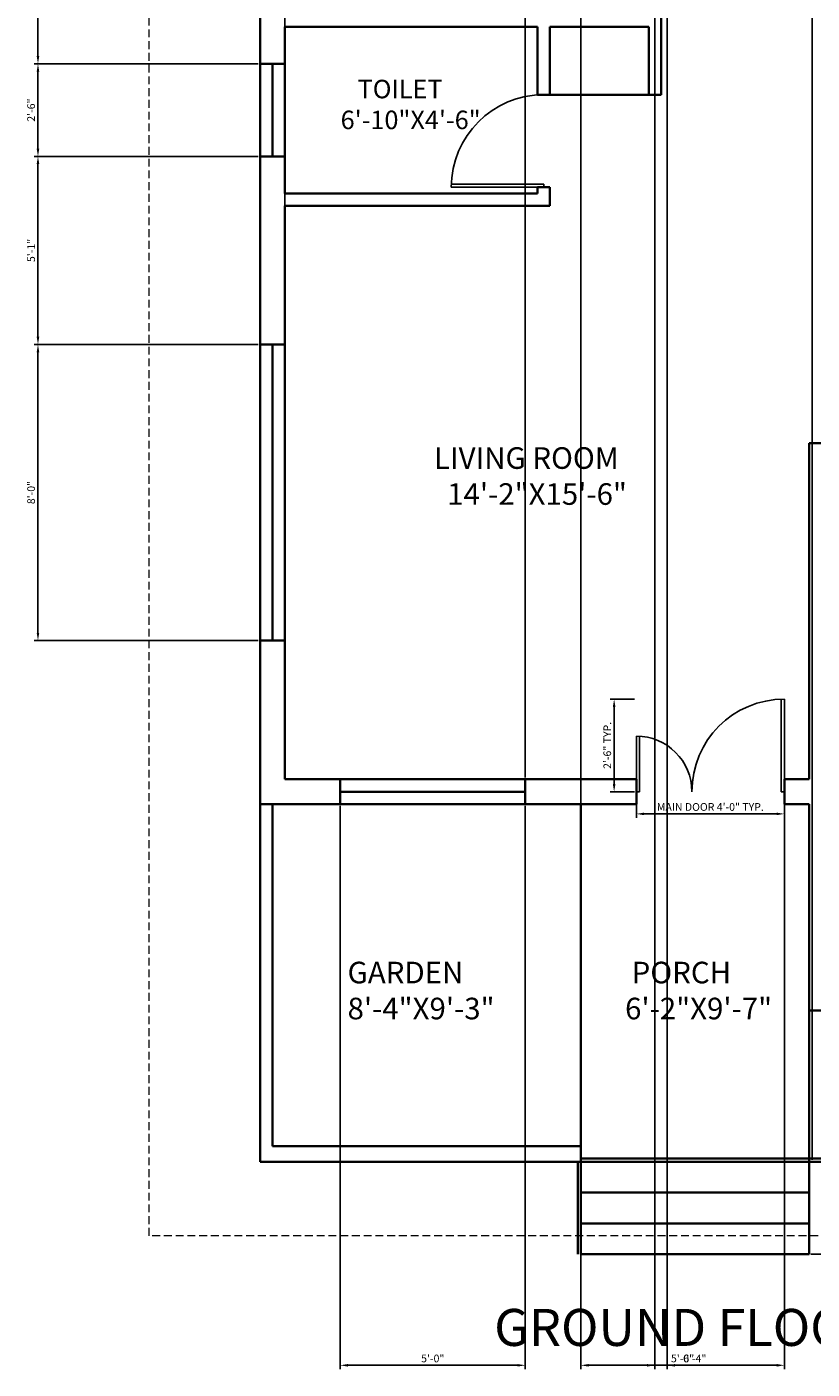
# Model space of a CAD drawing. Units: inches. Extents: x 1566 to 2546, y 1087 to 2705.
# Tile 24 of 27: x 1566 to 1821, y 1974 to 2409. Entities that reach past the tile are written whole.
import ezdxf

# ---------------------------------------------------------------- set-up
doc = ezdxf.new("R2010")
doc.units = ezdxf.units.IN
doc.linetypes.add('DASHED', pattern=[19.05, 12.7, -6.35])
for name, color, linetype, lineweight in [('A-ANNO-DIMS', 2, 'Continuous', 18), ('A-AREA-IDEN', 7, 'Continuous', 18), ('A-DOOR', 4, 'Continuous', 25), ('A-FLOR-OVHD', 8, 'DASHED', 18), ('A-WALL', 7, 'Continuous', 35)]:
    doc.layers.add(name, color=color, linetype=linetype, lineweight=lineweight)
doc.styles.get("Standard").update_dxf_attribs({"font": 'arial.ttf'})
doc.dimstyles.new('ISO-25', dxfattribs={"dimtxt": 2.5, "dimasz": 2.5, "dimexe": 1.25, "dimexo": 0.625, "dimtad": 1, "dimtxsty": 'Standard', "dimcen": 2.5, "dimadec": 0, "dimazin": 0, "dimtfac": 1, "dimtmove": 0, "dimatfit": 3, "dimfxl": 1, "dimarcsym": 0})

# ---------------------------------------------------------------- blocks, each defined once
blk = doc.blocks.new('d2')
for p, q in [((3364.08, 1632.29), (3364.08, 1602.29)), ((3365.08, 1632.29), (3365.08, 1602.29)), ((3364.08, 1602.29), (3365.08, 1602.29))]:
    blk.add_line(p, q)
at = {"ltscale": 0.3}
blk.add_arc((3364.08, 1602.29), 30, 0, 90, dxfattribs=at)
blk = doc.blocks.new('MD')
for p, q in [((1753.46, 1293.03), (1753.46, 1323.03)), ((1754.46, 1293.03), (1754.46, 1323.03)), ((1800.46, 1293.03), (1800.46, 1311.03)), ((1801.46, 1293.03), (1801.46, 1311.03)), ((1753.46, 1293.03), (1754.46, 1293.03)), ((1800.46, 1293.03), (1801.46, 1293.03))]:
    blk.add_line(p, q)
at = {"ltscale": 0.3}
for centre, radius, start, end in [((1753.46, 1293.03), 30, 0, 90), ((1801.46, 1293.03), 18, 90, 180)]:
    blk.add_arc(centre, radius, start, end, dxfattribs=at)
blk = doc.blocks.new('*D39')
at = {"layer": 'A-ANNO-DIMS', "color": 0, "lineweight": -2, "transparency": 16777216}
for p, q in [((1763.53, 2160.72), (1763.53, 2152.9)), ((1811.53, 2160.72), (1811.53, 2152.9)), ((1809.03, 2154.15), (1766.03, 2154.15))]:
    blk.add_line(p, q, dxfattribs=at)
at = {"layer": 'A-ANNO-DIMS', "color": 0, "transparency": 16777216}
for points in [[(1766.03, 2154.56), (1766.03, 2153.73), (1763.53, 2154.15)], [(1809.03, 2154.56), (1809.03, 2153.73), (1811.53, 2154.15)]]:
    blk.add_solid(points, dxfattribs=at)
at = {"layer": 'Defpoints', "color": 0, "transparency": 16777216}
for p in [(1763.53, 2161.35), (1811.53, 2161.35), (1763.53, 2154.15)]:
    blk.add_point(p, dxfattribs=at)
at = {"layer": 'A-ANNO-DIMS', "color": 0, "transparency": 16777216, "insert": (1787.53, 2156.07), "char_height": 2.5, "attachment_point": 5}
blk.add_mtext('MAIN DOOR 4\'-0" TYP.', dxfattribs=at)
blk = doc.blocks.new('*D40')
at = {"layer": 'A-ANNO-DIMS', "color": 0, "lineweight": -2, "transparency": 16777216}
for p, q in [((1762.9, 2191.35), (1755.08, 2191.35)), ((1756.33, 2163.85), (1756.33, 2188.85)), ((1762.9, 2161.35), (1755.08, 2161.35))]:
    blk.add_line(p, q, dxfattribs=at)
at = {"layer": 'A-ANNO-DIMS', "color": 0, "transparency": 16777216}
for points in [[(1755.91, 2188.85), (1756.75, 2188.85), (1756.33, 2191.35)], [(1755.91, 2163.85), (1756.75, 2163.85), (1756.33, 2161.35)]]:
    blk.add_solid(points, dxfattribs=at)
at = {"layer": 'Defpoints', "color": 0, "transparency": 16777216}
for p in [(1756.33, 2191.35), (1763.53, 2191.35), (1763.53, 2161.35)]:
    blk.add_point(p, dxfattribs=at)
at = {"layer": 'A-ANNO-DIMS', "color": 0, "transparency": 16777216, "insert": (1754.43, 2176.35), "char_height": 2.5, "attachment_point": 5, "rotation": 90}
blk.add_mtext('2\'-6" TYP.', dxfattribs=at)
blk = doc.blocks.new('*D70')
at = {"layer": 'A-ANNO-DIMS', "color": 0, "lineweight": -2, "transparency": 16777216}
for p, q in [((1769.53, 2656.72), (1769.53, 1974.1)), ((1773.53, 2656.72), (1773.53, 1974.1)), ((1767.03, 1975.35), (1764.53, 1975.35)), ((1769.53, 1975.35), (1773.53, 1975.35)), ((1776.03, 1975.35), (1786.43, 1975.35))]:
    blk.add_line(p, q, dxfattribs=at)
at = {"layer": 'A-ANNO-DIMS', "color": 0, "transparency": 16777216}
for points in [[(1767.03, 1975.76), (1767.03, 1974.93), (1769.53, 1975.35)], [(1776.03, 1975.76), (1776.03, 1974.93), (1773.53, 1975.35)]]:
    blk.add_solid(points, dxfattribs=at)
at = {"layer": 'Defpoints', "color": 0, "transparency": 16777216}
for p in [(1769.53, 2657.35), (1773.53, 2657.35), (1773.53, 1975.35)]:
    blk.add_point(p, dxfattribs=at)
at = {"layer": 'A-ANNO-DIMS', "color": 0, "transparency": 16777216, "insert": (1782.48, 1977.25), "char_height": 2.5, "attachment_point": 5}
blk.add_mtext('0\'-4"', dxfattribs=at)
blk = doc.blocks.new('*D75')
at = {"layer": 'A-ANNO-DIMS', "color": 0, "lineweight": -2, "transparency": 16777216}
for p, q in [((1640.9, 2437.35), (1568.28, 2437.35)), ((1569.53, 2434.85), (1569.53, 2399.85)), ((1640.9, 2397.35), (1568.28, 2397.35))]:
    blk.add_line(p, q, dxfattribs=at)
at = {"layer": 'A-ANNO-DIMS', "color": 0, "transparency": 16777216}
for points in [[(1569.11, 2434.85), (1569.95, 2434.85), (1569.53, 2437.35)], [(1569.11, 2399.85), (1569.95, 2399.85), (1569.53, 2397.35)]]:
    blk.add_solid(points, dxfattribs=at)
at = {"layer": 'Defpoints', "color": 0, "transparency": 16777216}
for p in [(1641.53, 2437.35), (1569.53, 2397.35), (1641.53, 2397.35)]:
    blk.add_point(p, dxfattribs=at)
at = {"layer": 'A-ANNO-DIMS', "color": 0, "transparency": 16777216, "insert": (1567.63, 2417.35), "char_height": 2.5, "attachment_point": 5, "rotation": 90}
blk.add_mtext('3\'-4"', dxfattribs=at)
blk = doc.blocks.new('*D76')
at = {"layer": 'A-ANNO-DIMS', "color": 0, "lineweight": -2, "transparency": 16777216}
for p, q in [((1640.9, 2397.35), (1568.28, 2397.35)), ((1569.53, 2394.85), (1569.53, 2369.85)), ((1640.9, 2367.35), (1568.28, 2367.35))]:
    blk.add_line(p, q, dxfattribs=at)
at = {"layer": 'A-ANNO-DIMS', "color": 0, "transparency": 16777216}
for points in [[(1569.11, 2394.85), (1569.95, 2394.85), (1569.53, 2397.35)], [(1569.11, 2369.85), (1569.95, 2369.85), (1569.53, 2367.35)]]:
    blk.add_solid(points, dxfattribs=at)
at = {"layer": 'Defpoints', "color": 0, "transparency": 16777216}
for p in [(1641.53, 2397.35), (1569.53, 2367.35), (1641.53, 2367.35)]:
    blk.add_point(p, dxfattribs=at)
at = {"layer": 'A-ANNO-DIMS', "color": 0, "transparency": 16777216, "insert": (1567.63, 2382.35), "char_height": 2.5, "attachment_point": 5, "rotation": 90}
blk.add_mtext('2\'-6"', dxfattribs=at)
blk = doc.blocks.new('*D77')
at = {"layer": 'A-ANNO-DIMS', "color": 0, "lineweight": -2, "transparency": 16777216}
for p, q in [((1640.9, 2367.35), (1568.28, 2367.35)), ((1569.53, 2364.85), (1569.53, 2308.85)), ((1640.9, 2306.35), (1568.28, 2306.35))]:
    blk.add_line(p, q, dxfattribs=at)
at = {"layer": 'A-ANNO-DIMS', "color": 0, "transparency": 16777216}
for points in [[(1569.11, 2364.85), (1569.95, 2364.85), (1569.53, 2367.35)], [(1569.11, 2308.85), (1569.95, 2308.85), (1569.53, 2306.35)]]:
    blk.add_solid(points, dxfattribs=at)
at = {"layer": 'Defpoints', "color": 0, "transparency": 16777216}
for p in [(1641.53, 2367.35), (1569.53, 2306.35), (1641.53, 2306.35)]:
    blk.add_point(p, dxfattribs=at)
at = {"layer": 'A-ANNO-DIMS', "color": 0, "transparency": 16777216, "insert": (1567.63, 2336.85), "char_height": 2.5, "attachment_point": 5, "rotation": 90}
blk.add_mtext('5\'-1"', dxfattribs=at)
blk = doc.blocks.new('*D78')
at = {"layer": 'A-ANNO-DIMS', "color": 0, "lineweight": -2, "transparency": 16777216}
for p, q in [((1640.9, 2306.35), (1568.28, 2306.35)), ((1569.53, 2303.85), (1569.53, 2212.85)), ((1640.9, 2210.35), (1568.28, 2210.35))]:
    blk.add_line(p, q, dxfattribs=at)
at = {"layer": 'A-ANNO-DIMS', "color": 0, "transparency": 16777216}
for points in [[(1569.11, 2303.85), (1569.95, 2303.85), (1569.53, 2306.35)], [(1569.11, 2212.85), (1569.95, 2212.85), (1569.53, 2210.35)]]:
    blk.add_solid(points, dxfattribs=at)
at = {"layer": 'Defpoints', "color": 0, "transparency": 16777216}
for p in [(1641.53, 2306.35), (1569.53, 2210.35), (1641.53, 2210.35)]:
    blk.add_point(p, dxfattribs=at)
at = {"layer": 'A-ANNO-DIMS', "color": 0, "transparency": 16777216, "insert": (1567.63, 2258.35), "char_height": 2.5, "attachment_point": 5, "rotation": 90}
blk.add_mtext('8\'-0"', dxfattribs=at)
blk = doc.blocks.new('*D79')
at = {"layer": 'A-ANNO-DIMS', "color": 0, "lineweight": -2, "transparency": 16777216}
for p, q in [((1649.53, 2165.97), (1649.53, 2702.6)), ((1652.03, 2701.35), (1725.03, 2701.35)), ((1727.53, 2165.97), (1727.53, 2702.6))]:
    blk.add_line(p, q, dxfattribs=at)
at = {"layer": 'A-ANNO-DIMS', "color": 0, "transparency": 16777216}
for points in [[(1652.03, 2701.76), (1652.03, 2700.93), (1649.53, 2701.35)], [(1725.03, 2701.76), (1725.03, 2700.93), (1727.53, 2701.35)]]:
    blk.add_solid(points, dxfattribs=at)
at = {"layer": 'Defpoints', "color": 0, "transparency": 16777216}
for p in [(1727.53, 2701.35), (1649.53, 2165.35), (1727.53, 2165.35)]:
    blk.add_point(p, dxfattribs=at)
at = {"layer": 'A-ANNO-DIMS', "color": 0, "transparency": 16777216, "insert": (1688.53, 2703.25), "char_height": 2.5, "attachment_point": 5}
blk.add_mtext('6\'-6"', dxfattribs=at)
blk = doc.blocks.new('*D80')
at = {"layer": 'A-ANNO-DIMS', "color": 0, "lineweight": -2, "transparency": 16777216}
for p, q in [((1667.53, 2156.72), (1667.53, 1974.1)), ((1727.53, 2156.72), (1727.53, 1974.1)), ((1670.03, 1975.35), (1725.03, 1975.35))]:
    blk.add_line(p, q, dxfattribs=at)
at = {"layer": 'A-ANNO-DIMS', "color": 0, "transparency": 16777216}
for points in [[(1670.03, 1975.76), (1670.03, 1974.93), (1667.53, 1975.35)], [(1725.03, 1975.76), (1725.03, 1974.93), (1727.53, 1975.35)]]:
    blk.add_solid(points, dxfattribs=at)
at = {"layer": 'Defpoints', "color": 0, "transparency": 16777216}
for p in [(1667.53, 2157.35), (1727.53, 2157.35), (1727.53, 1975.35)]:
    blk.add_point(p, dxfattribs=at)
at = {"layer": 'A-ANNO-DIMS', "color": 0, "transparency": 16777216, "insert": (1697.53, 1977.25), "char_height": 2.5, "attachment_point": 5}
blk.add_mtext('5\'-0"', dxfattribs=at)
blk = doc.blocks.new('*D86')
at = {"layer": 'A-ANNO-DIMS', "color": 0, "lineweight": -2, "transparency": 16777216}
for p, q in [((1745.53, 2041.97), (1745.53, 2702.6)), ((1748.03, 2701.35), (1818.03, 2701.35)), ((1820.53, 2041.97), (1820.53, 2702.6))]:
    blk.add_line(p, q, dxfattribs=at)
at = {"layer": 'A-ANNO-DIMS', "color": 0, "transparency": 16777216}
for points in [[(1748.03, 2701.76), (1748.03, 2700.93), (1745.53, 2701.35)], [(1818.03, 2701.76), (1818.03, 2700.93), (1820.53, 2701.35)]]:
    blk.add_solid(points, dxfattribs=at)
at = {"layer": 'Defpoints', "color": 0, "transparency": 16777216}
for p in [(1820.53, 2701.35), (1745.53, 2041.35), (1820.53, 2041.35)]:
    blk.add_point(p, dxfattribs=at)
at = {"layer": 'A-ANNO-DIMS', "color": 0, "transparency": 16777216, "insert": (1783.03, 2703.25), "char_height": 2.5, "attachment_point": 5}
blk.add_mtext('6\'-3"', dxfattribs=at)
blk = doc.blocks.new('*D87')
at = {"layer": 'A-ANNO-DIMS', "color": 0, "lineweight": -2, "transparency": 16777216}
for p, q in [((1821.15, 2041.35), (2038.78, 2041.35)), ((2037.53, 2038.85), (2037.53, 2013.85)), ((1820.15, 2011.35), (2038.78, 2011.35))]:
    blk.add_line(p, q, dxfattribs=at)
at = {"layer": 'A-ANNO-DIMS', "color": 0, "transparency": 16777216}
for points in [[(2037.11, 2038.85), (2037.95, 2038.85), (2037.53, 2041.35)], [(2037.11, 2013.85), (2037.95, 2013.85), (2037.53, 2011.35)]]:
    blk.add_solid(points, dxfattribs=at)
at = {"layer": 'Defpoints', "color": 0, "transparency": 16777216}
for p in [(1820.53, 2041.35), (1819.53, 2011.35), (2037.53, 2011.35)]:
    blk.add_point(p, dxfattribs=at)
at = {"layer": 'A-ANNO-DIMS', "color": 0, "transparency": 16777216, "insert": (2035.63, 2026.35), "char_height": 2.5, "attachment_point": 5, "rotation": 90}
blk.add_mtext('2\'-6"', dxfattribs=at)
blk = doc.blocks.new('*D88')
at = {"layer": 'A-ANNO-DIMS', "color": 0, "lineweight": -2, "transparency": 16777216}
for p, q in [((1745.53, 2156.72), (1745.53, 1974.1)), ((1811.53, 2156.72), (1811.53, 1974.1)), ((1748.03, 1975.35), (1809.03, 1975.35))]:
    blk.add_line(p, q, dxfattribs=at)
at = {"layer": 'A-ANNO-DIMS', "color": 0, "transparency": 16777216}
for points in [[(1748.03, 1975.76), (1748.03, 1974.93), (1745.53, 1975.35)], [(1809.03, 1975.76), (1809.03, 1974.93), (1811.53, 1975.35)]]:
    blk.add_solid(points, dxfattribs=at)
at = {"layer": 'Defpoints', "color": 0, "transparency": 16777216}
for p in [(1745.53, 2157.35), (1811.53, 2157.35), (1811.53, 1975.35)]:
    blk.add_point(p, dxfattribs=at)
at = {"layer": 'A-ANNO-DIMS', "color": 0, "transparency": 16777216, "insert": (1778.53, 1977.25), "char_height": 2.5, "attachment_point": 5}
blk.add_mtext('5\'-6"', dxfattribs=at)

msp = doc.modelspace()

# ---------------------------------------------------------------- linework, layer by layer
at = {"layer": 'A-FLOR-OVHD', "ltscale": 0.2}
for p, q in [((1605.53, 2017.35), (1605.53, 2665.35)), ((2001.53, 2017.35), (1605.53, 2017.35))]:
    msp.add_line(p, q, dxfattribs=at)
at = {"layer": 'A-WALL'}
for p, q in [((1641.53, 2041.35), (1641.53, 2665.35)), ((1771.53, 2387.35), (1771.53, 2413.35)), ((1649.53, 2355.35), (1649.53, 2409.35)), ((1649.53, 2409.35), (1731.53, 2409.35)), ((1731.53, 2387.35), (1731.53, 2409.35)), ((1735.53, 2409.35), (1767.53, 2409.35)), ((1735.53, 2387.35), (1735.53, 2409.35)), ((1767.53, 2387.35), (1767.53, 2409.35)), ((1649.53, 2397.35), (1641.53, 2397.35)), ((1645.53, 2397.35), (1645.53, 2367.35)), ((1731.53, 2387.35), (1771.53, 2387.35)), ((1649.53, 2367.35), (1641.53, 2367.35)), ((1649.53, 2355.35), (1731.53, 2355.35)), ((1731.53, 2355.35), (1731.53, 2357.35)), ((1731.53, 2357.35), (1735.53, 2357.35)), ((1735.53, 2351.35), (1735.53, 2357.35)), ((1649.53, 2165.35), (1649.53, 2351.35)), ((1649.53, 2351.35), (1735.53, 2351.35)), ((1649.53, 2306.35), (1641.53, 2306.35)), ((1645.53, 2306.35), (1645.53, 2210.35)), ((1819.53, 2274.35), (1827.53, 2274.35)), ((1819.53, 2165.35), (1819.53, 2274.35)), ((1649.53, 2210.35), (1641.53, 2210.35)), ((1649.53, 2165.35), (1763.53, 2165.35)), ((1667.53, 2157.35), (1667.53, 2165.35)), ((1727.53, 2157.35), (1727.53, 2165.35)), ((1763.53, 2157.35), (1763.53, 2165.35)), ((1811.53, 2157.35), (1811.53, 2165.35)), ((1811.53, 2165.35), (1819.53, 2165.35)), ((1727.53, 2161.35), (1667.53, 2161.35)), ((1641.53, 2157.35), (1763.53, 2157.35)), ((1645.53, 2046.35), (1645.53, 2157.35)), ((1745.53, 2041.35), (1745.53, 2157.35)), ((1811.53, 2157.35), (1819.53, 2157.35)), ((1819.53, 2042.35), (1819.53, 2157.35)), ((1819.53, 2090.35), (1993.53, 2090.35)), ((1645.53, 2046.35), (1745.53, 2046.35)), ((2001.53, 2041.35), (1641.53, 2041.35)), ((1744.53, 2041.35), (1744.53, 2011.35)), ((1993.53, 2042.35), (1745.53, 2042.35)), ((1745.53, 2041.35), (1745.53, 2011.35)), ((1819.53, 2042.35), (1819.53, 2011.35)), ((1819.53, 2031.35), (1745.53, 2031.35)), ((1819.53, 2021.35), (1745.53, 2021.35)), ((1819.53, 2011.35), (1745.53, 2011.35))]:
    msp.add_line(p, q, dxfattribs=at)

# ---------------------------------------------------------------- block references
at = {"layer": 'A-DOOR', "rotation": 90}
msp.add_blockref('d2', (3335.82, -1006.73), dxfattribs=at)
at = {"layer": 'A-DOOR', "xscale": -1}
msp.add_blockref('MD', (3564.99, 868.32), dxfattribs=at)

# ---------------------------------------------------------------- texts
at = {"layer": 'A-AREA-IDEN', "attachment_point": 1}
for s, width, insert, char_height in [('   TOILET\\P6\'-10"X4\'-6"', 111.7553, (1667.66, 2392.18), 6), ('LIVING ROOM\\P  14\'-2"X15\'-6"', 111.7553, (1697.93, 2273.03), 7), ('GARDEN\\P8\'-4"X9\'-3"', 111.7553, (1669.9, 2106.2), 7), (' PORCH\\P6\'-2"X9\'-7"', 111.7553, (1759.88, 2106.2), 7), ('GROUND FLOOR PLAN', 267.5424, (1717.44, 1993.63), 12)]:
    msp.add_mtext_dynamic_manual_height_columns(s, width=width, gutter_width=12.5, heights=[0], dxfattribs=dict(at, insert=insert, char_height=char_height))

# ---------------------------------------------------------------- dimensions: what is measured, and where the dimension line sits
at = {"layer": 'A-ANNO-DIMS'}
for base, p1, p2, picture, middle in [((1727.53, 2701.35), (1649.53, 2165.35), (1727.53, 2165.35), '*D79', (1688.53, 2703.25)), ((1820.53, 2701.35), (1745.53, 2041.35), (1820.53, 2041.35), '*D86', (1783.03, 2703.25)), ((1773.53, 1975.35), (1769.53, 2657.35), (1773.53, 2657.35), '*D70', (1782.48, 1977.25)), ((1727.53, 1975.35), (1667.53, 2157.35), (1727.53, 2157.35), '*D80', (1697.53, 1977.25)), ((1811.53, 1975.35), (1745.53, 2157.35), (1811.53, 2157.35), '*D88', (1778.53, 1977.25))]:
    dim = msp.add_linear_dim(base=base, p1=p1, p2=p2, dimstyle='ISO-25', override={"dimdec": 1, "dimlfac": 1, "dimrnd": 0, "dimzin": 1, "dimdsep": 46, "dimlunit": 4, "dimfrac": 2}, dxfattribs=at)
    dim.commit()
    dim.dimension.update_dxf_attribs({"geometry": picture, "text_midpoint": middle})
for base, p1, p2, picture, middle in [((1569.53, 2397.35), (1641.53, 2437.35), (1641.53, 2397.35), '*D75', (1567.63, 2417.35)), ((1569.53, 2367.35), (1641.53, 2397.35), (1641.53, 2367.35), '*D76', (1567.63, 2382.35)), ((1569.53, 2306.35), (1641.53, 2367.35), (1641.53, 2306.35), '*D77', (1567.63, 2336.85)), ((1569.53, 2210.35), (1641.53, 2306.35), (1641.53, 2210.35), '*D78', (1567.63, 2258.35)), ((2037.53, 2011.35), (1820.53, 2041.35), (1819.53, 2011.35), '*D87', (2035.63, 2026.35))]:
    dim = msp.add_linear_dim(base=base, p1=p1, p2=p2, angle=90, dimstyle='ISO-25', override={"dimdec": 1, "dimlfac": 1, "dimrnd": 0, "dimzin": 1, "dimdsep": 46, "dimlunit": 4, "dimfrac": 2}, dxfattribs=at)
    dim.commit()
    dim.dimension.update_dxf_attribs({"geometry": picture, "text_midpoint": middle})
for base, p1, p2, angle, text, picture, middle in [((1756.33, 2191.35), (1763.53, 2161.35), (1763.53, 2191.35), 90, '<> TYP.', '*D40', (1754.43, 2176.35)), ((1763.53, 2154.15), (1811.53, 2161.35), (1763.53, 2161.35), 180, 'MAIN DOOR <> TYP.', '*D39', (1787.53, 2156.07))]:
    dim = msp.add_linear_dim(base=base, p1=p1, p2=p2, angle=angle, text=text, dimstyle='ISO-25', override={"dimdec": 1, "dimrnd": 0, "dimzin": 1, "dimlunit": 4, "dimfrac": 2}, dxfattribs=at)
    dim.commit()
    dim.dimension.update_dxf_attribs({"geometry": picture, "text_midpoint": middle})

doc.saveas('drawing.dxf')
